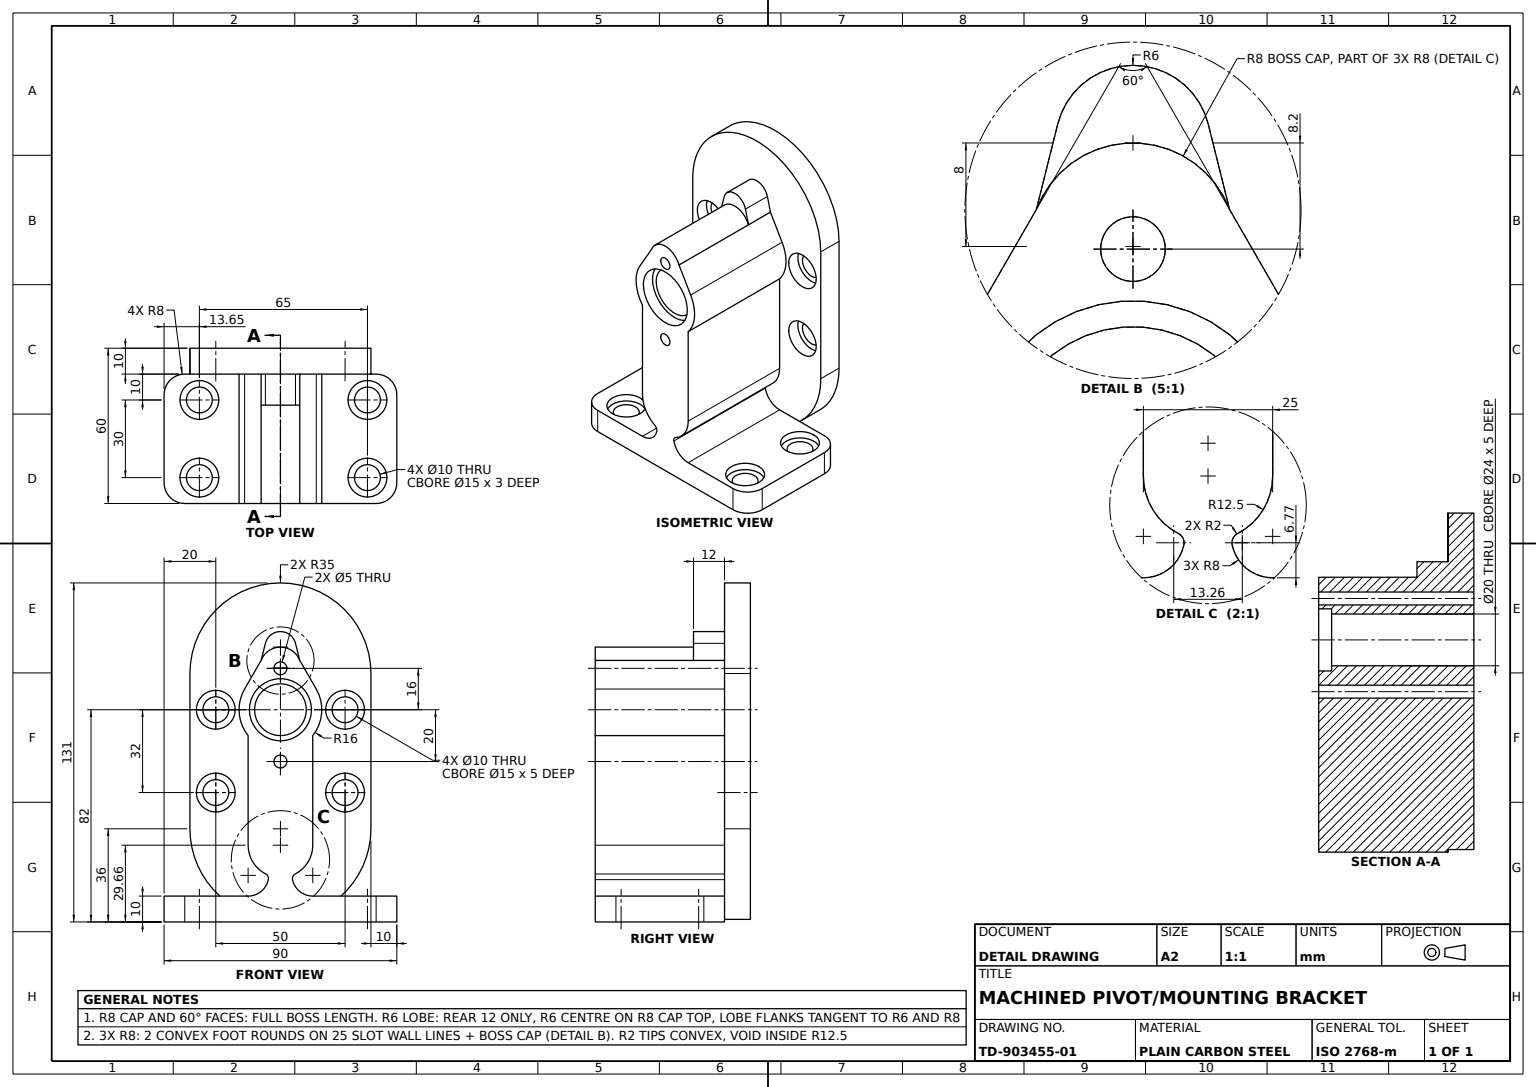
SolidWorks part; units mm, degrees
material "Plain Carbon Steel"
ref_plane "Front Plane" through (0, 0, 0) normal (0, 0, 1) x (1, 0, 0)
ref_plane "Top Plane" through (0, 0, 0) normal (0, 1, 0) x (1, 0, 0)
ref_plane "Right Plane" through (0, 0, 0) normal (1, 0, 0) x (0, 0, -1)
sketch "Flange Plate Sketch" plane through (0, 0, 0) normal (0, 0, 1) x (1, 0, 0)
  line L3 (-35, -46) -> (-35, 14)
  line L5 (35, -46) -> (35, 14)
  line L6 (-35, -46) -> (35, 14) construction
  line L7 (-35, 14) -> (35, -46) construction
  circle A0 centre (-25, 0) radius 5
  circle A1 centre (25, 0) radius 5
  circle A2 centre (-25, -32) radius 5
  circle A3 centre (25, -32) radius 5
  arc A4 (-35, 14) -> (35, 14) centre (0, 14) cw
  arc A5 (-35, -46) -> (35, -46) centre (0, -46) ccw
  point P11 (0, -16)
  dimension "D1" = 32
  dimension "D8" = 35
  dimension "D10" = 10
  dimension "D11" = 10
  dimension "D12" = 10
  dimension "D13" = 10
  dimension "D2" = 50
  dimension "D3" = 25
  dimension "D4" = 32
  dimension "D5" = 50
  dimension "D6" = 25
  dimension "D7" = 25
  dimension "D9" = 60
  dimension "D14" = 14
extrude "Flange Plate" add sketch "Flange Plate Sketch" along normal blind 10
sketch "Flange Recess Sketch" plane through (0, 0, 10) normal (0, 0, 1) x (1, 0, 0)
  circle A0 centre (-25, 0) radius 7.5
  circle A1 centre (25, 0) radius 7.5
  circle A2 centre (25, -32) radius 7.5
  circle A3 centre (-25, -32) radius 7.5
  circle A4 centre (-25, 0) radius 5
  circle A5 centre (25, 0) radius 5
  circle A6 centre (25, -32) radius 5
  circle A7 centre (-25, -32) radius 5
  dimension "D1" = 15
  dimension "D2" = 15
  dimension "D3" = 15
  dimension "D4" = 15
  dimension "D5" = 10
  dimension "D6" = 10
  dimension "D7" = 10
  dimension "D8" = 10
extrude "Flange Recess 5mm" cut sketch "Flange Recess Sketch" against normal blind 5
sketch "Bracket Body Sketch" plane through (0, 0, 10) normal (0, 0, 1) x (1, 0, 0)
  line L0 (-45, -82) -> (45, -82)
  line L1 (-7.4734, 19.0557) -> (-13.8564, 8)
  line L4 (45, -82) -> (45, -72)
  line L5 (7.4734, 19.0557) -> (13.8564, 8)
  line L6 (0, 0) -> (0, -10)
  line L7 (-12.5, -9.9875) -> (-12.5, -52.3381)
  line L8 (12.5, -9.9875) -> (12.5, -52.3381)
  line L9 (45, -72) -> (12.5, -72)
  line L12 (-45, -72) -> (-45, -82)
  line L16 (-12.5, -72) -> (-45, -72)
  circle A0 centre (0, 0) radius 10
  arc A1 (-13.8564, 8) -> (-12.5, -9.9875) centre (0, 0) ccw
  circle A2 centre (0, 16) radius 2.5
  arc A5 (12.5, -9.9875) -> (13.8564, 8) centre (0, 0) ccw
  arc A7 (-7.4734, 19.0557) -> (7.4734, 19.0557) centre (0, 16.2012) cw
  arc A8 (-12.5, -52.3381) -> (-5.7141, -63.4556) centre (0, -52.3381) ccw
  arc A9 (-12.5, -72) -> (-4.6711, -65.6459) centre (-12.5, -64) ccw
  arc A10 (-5.7141, -63.4556) -> (-4.6711, -65.6459) centre (-6.6284, -65.2344) cw
  arc A11 (12.5, -72) -> (4.6711, -65.6459) centre (12.5, -64) cw
  arc A12 (12.5, -52.3381) -> (5.7141, -63.4556) centre (0, -52.3381) cw
  arc A13 (5.7141, -63.4556) -> (4.6711, -65.6459) centre (6.6284, -65.2344) ccw
  circle A14 centre (0, -20) radius 2.5
  circle A15 centre (25, 0) radius 7.5 construction
  point P3 (0, -90)
  point P9 (0, -82)
  point P17 (0, -82)
  point P18 (-12.5, 0)
  point P19 (-12.5, -90)
  point P20 (12.5, 0)
  point P21 (12.5, -90)
  point P32 (-4.5, -64)
  arc M21 (-35, -46) -> (35, -46) centre (0, -46) ccw
  dimension "D1" = 32
  dimension "D2" = 20
  dimension "D3" = 10
  dimension "D4" = 90
  dimension "D5" = 5
  dimension "D10" = 12.5
  dimension "D11" = 2
  dimension "D8" = 36
  dimension "D9" = 5
  dimension "D12" = 8
  dimension "D6" = 82
  dimension "D7" = 45
  dimension "D13" = 20
  dimension "D14" = 11.1436
  dimension "D15" = 17.5266
  dimension "D16" = 8
  dimension "D17" = 10
extrude "Bracket Body" add sketch "Bracket Body Sketch" along normal blind 50 contours A13 A12 L8 A5 L5 A7 L1 A1 L7 A8 A10 A9 L16 L9 A11 A14 A2 A0 M21 | L16 L12 L0 L4 L9 M21
sketch "Through Bore Sketch" plane through (0, 0, 10) normal (0, 0, 1) x (1, 0, 0)
  circle A0 centre (0, 0) radius 10
  dimension "D1" = 20
extrude "Through Bore" cut sketch "Through Bore Sketch" against normal blind 50
sketch "Bore Counterbore Sketch" plane through (0, 0, 60) normal (0, 0, 1) x (1, 0, 0)
  circle A0 centre (0, 0) radius 12
  dimension "D1" = 24
extrude "Bore Counterbore Ø24" cut sketch "Bore Counterbore Sketch" against normal blind 5
sketch "Body Pocket Sketch" plane through (0, -72, 0) normal (0, 1, 0) x (1, 0, 0)
  line L0 (-23.4307, -10) -> (-45, -10) construction
  line L1 (-45, -60) -> (-45, -10) construction
  line L2 (-12.5, -60) -> (-45, -60) construction
  line L4 (45, -60) -> (12.5, -60) construction
  line L5 (45, -10) -> (23.4307, -10) construction
  circle A0 centre (-31.3503, -20) radius 5
  circle A1 centre (-31.3503, -50) radius 5
  circle A2 centre (33.6497, -20) radius 5
  circle A3 centre (33.6497, -50) radius 5
  dimension "D1" = 10
  dimension "D2" = 10
  dimension "D3" = 10
  dimension "D4" = 10
  dimension "D5" = 10
  dimension "D6" = 10
  dimension "D7" = 30
  dimension "D8" = 10
  dimension "D9" = 10
  dimension "D10" = 65
  dimension "D11" = 65
  dimension "D12" = 13.6497
extrude "Body Pocket 20mm" cut sketch "Body Pocket Sketch" against normal blind 20
sketch "Pocket Step Sketch" plane through (0, -72, 0) normal (0, 1, 0) x (1, 0, 0)
  circle A0 centre (-31.3503, -20) radius 7.5
  circle A1 centre (-31.3503, -50) radius 7.5
  circle A2 centre (33.6497, -20) radius 7.5
  circle A3 centre (33.6497, -50) radius 7.5
  dimension "D1" = 15
extrude "Pocket Step 3mm" cut sketch "Pocket Step Sketch" against normal blind 3
sketch "Body Boss Sketch" plane through (0, 0, 10) normal (0, 0, 1) x (1, 0, 0)
  line L0 (7.4734, 19.0557) -> (5.8204, 25.6583)
  line L1 (-7.4734, 19.0557) -> (-5.8204, 25.6583)
  arc A0 (5.8204, 25.6583) -> (-5.8204, 25.6583) centre (0, 24.2012) ccw
  arc A1 (7.4734, 19.0557) -> (-7.4734, 19.0557) centre (0, 16.2012) ccw construction
  arc A2 (-7.4734, 19.0557) -> (7.4734, 19.0557) centre (0, 16.2012) cw
  dimension "D1" = 12
extrude "Body Boss 12mm" add sketch "Body Boss Sketch" along normal blind 12
fillet "Body Fillet R8 A" radius 8 2 edges at (45, -77, 60) (-45, -77, 60)
fillet "Body Fillet R8 B" radius 8 2 edges at (-45, -77, 10) (45, -77, 10)
sketch "Body Slot Sketch" plane through (0, 0, 60) normal (0, 0, 1) x (1, 0, 0)
  circle A0 centre (0, 16) radius 2.5
  circle A1 centre (0, -20) radius 2.5
  dimension "D1" = 5
extrude "Body Slot Cut" cut sketch "Body Slot Sketch" against normal through all
